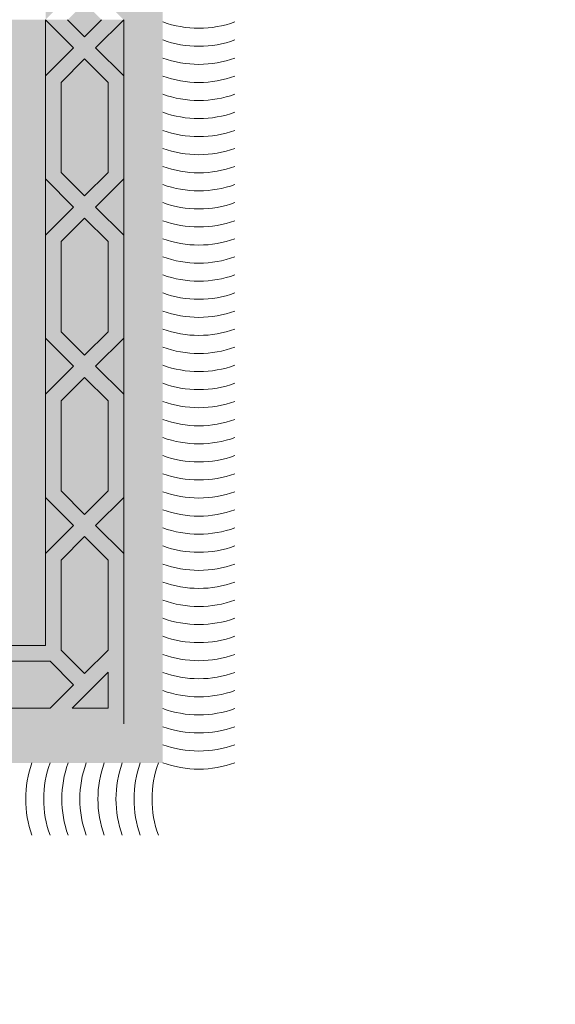
# Model space of a CAD drawing. Units: inches. Extents: x 844 to 2234, y 346 to 1084.
# Tile 12 of 93: x 1127.54 to 1136.28, y 680.17 to 696.22. Entities that reach past the tile are written whole.
import ezdxf

# ---------------------------------------------------------------- set-up
doc = ezdxf.new("R2010")
doc.units = ezdxf.units.IN
doc.header["$MEASUREMENT"] = 0
for name, color, linetype, lineweight in [('A-ANNO-DIMS', 2, 'Continuous', 18), ('furniture', 8, 'Continuous', 18), ('RA-AP-01$0$INT', 35, 'Continuous', 5)]:
    doc.layers.add(name, color=color, linetype=linetype, lineweight=lineweight)
doc.layers.add('RA-AP-01$0$FURN', color=3, linetype='Continuous')
doc.styles.get("Standard").update_dxf_attribs({"font": 'arial.ttf'})
doc.dimstyles.get("Standard").update_dxf_attribs({"dimtxt": 6, "dimasz": 3, "dimexe": 0.18, "dimexo": 0.0625, "dimgap": 0.09, "dimtad": 0, "dimtih": 1, "dimtoh": 1, "dimdec": 1, "dimzin": 0, "dimdsep": 46, "dimlunit": 3, "dimtxsty": 'Standard', "dimblk": 'ARCHTICK', "dimcen": 0.09, "dimadec": 0, "dimazin": 0, "dimtfac": 1, "dimtdec": 1, "dimtofl": 0, "dimtmove": 0, "dimatfit": 3, "dimfxl": 1, "dimtolj": 1, "dimtzin": 0, "dimarcsym": 0})

# ---------------------------------------------------------------- blocks, each defined once
blk = doc.blocks.new('A$C18D01794')
at = {"layer": 'RA-AP-01$0$INT'}
h = blk.add_hatch(color=256, dxfattribs=at)
h.paths.add_polyline_path([(4.3552, -6.1567), (4.3552, -8.0567), (5.4552, -8.0567), (5.4552, -6.1567)])
h.paths.add_polyline_path([(4.4052, -8.0067), (4.4052, -6.2067), (5.4052, -6.2067), (5.4052, -8.0067)], flags=16)
h = blk.add_hatch(color=256, dxfattribs=at)
h.paths.add_polyline_path([(4.4693, -7.0709), (4.5052, -7.035), (4.5052, -7.1067)])
h.paths.add_polyline_path([(4.4552, -7.085), (4.4769, -7.1067), (4.4335, -7.1067)])
h.paths.add_polyline_path([(4.4052, -7.035), (4.4411, -7.0709), (4.4052, -7.1067)])
h.paths.add_polyline_path([(4.4252, -6.9115), (4.4552, -6.8815), (4.4852, -6.9115), (4.4852, -7.0267), (4.4552, -7.0567), (4.4252, -7.0267)])
h.paths.add_polyline_path([(4.5052, -6.8315), (4.5052, -6.9032), (4.4693, -6.8673)])
h.paths.add_polyline_path([(4.4252, -6.7079), (4.4552, -6.6779), (4.4852, -6.7079), (4.4852, -6.8232), (4.4552, -6.8532), (4.4252, -6.8232)])
h.paths.add_polyline_path([(4.4252, -6.5044), (4.4552, -6.4744), (4.4852, -6.5044), (4.4852, -6.6196), (4.4552, -6.6496), (4.4252, -6.6196)])
h.paths.add_polyline_path([(4.4693, -6.6638), (4.5052, -6.6279), (4.5052, -6.6996)])
h.paths.add_polyline_path([(4.4052, -6.6279), (4.4411, -6.6638), (4.4052, -6.6996)])
h.paths.add_polyline_path([(4.4052, -6.4244), (4.4411, -6.4602), (4.4052, -6.4961)])
h.paths.add_polyline_path([(4.4693, -6.4602), (4.5052, -6.4244), (4.5052, -6.4961)])
h.paths.add_polyline_path([(4.4252, -6.3009), (4.4552, -6.2709), (4.4852, -6.3009), (4.4852, -6.4161), (4.4552, -6.4461), (4.4252, -6.4161)])
h.paths.add_polyline_path([(4.4252, -6.2267), (4.4711, -6.2267), (4.4252, -6.2726)])
h.paths.add_polyline_path([(4.4993, -6.2267), (4.6361, -6.2267), (4.6661, -6.2567), (4.6361, -6.2867), (4.4993, -6.2867), (4.4693, -6.2567)])
h.paths.add_polyline_path([(4.6802, -6.2709), (4.7161, -6.3067), (4.6443, -6.3067)])
h.paths.add_polyline_path([(4.6443, -6.2067), (4.7161, -6.2067), (4.6802, -6.2426)])
h.paths.add_polyline_path([(4.7243, -6.2267), (4.8611, -6.2267), (4.8911, -6.2567), (4.8611, -6.2867), (4.7243, -6.2867), (4.6943, -6.2567)])
h.paths.add_polyline_path([(4.9052, -6.2709), (4.9411, -6.3067), (4.8693, -6.3067)])
h.paths.add_polyline_path([(4.8693, -6.2067), (4.9411, -6.2067), (4.9052, -6.2426)])
h.paths.add_polyline_path([(4.9493, -6.2267), (5.0861, -6.2267), (5.1161, -6.2567), (5.0861, -6.2867), (4.9493, -6.2867), (4.9193, -6.2567)])
h.paths.add_polyline_path([(5.1302, -6.2709), (5.1661, -6.3067), (5.0943, -6.3067)])
h.paths.add_polyline_path([(5.0943, -6.2067), (5.1661, -6.2067), (5.1302, -6.2426)])
h.paths.add_polyline_path([(5.1743, -6.2267), (5.3111, -6.2267), (5.3411, -6.2567), (5.3111, -6.2867), (5.1743, -6.2867), (5.1443, -6.2567)])
h.paths.add_polyline_path([(5.3252, -6.3009), (5.3552, -6.2709), (5.3852, -6.3009), (5.3852, -6.4161), (5.3552, -6.4461), (5.3252, -6.4161)])
h.paths.add_polyline_path([(5.3393, -6.2267), (5.3852, -6.2267), (5.3852, -6.2726)])
h.paths.add_polyline_path([(5.3252, -6.5044), (5.3552, -6.4744), (5.3852, -6.5044), (5.3852, -6.6196), (5.3552, -6.6496), (5.3252, -6.6196)])
h.paths.add_polyline_path([(5.3052, -6.4244), (5.3411, -6.4602), (5.3052, -6.4961)])
h.paths.add_polyline_path([(5.3693, -6.4602), (5.4052, -6.4244), (5.4052, -6.4961)])
h.paths.add_polyline_path([(5.4052, -6.6279), (5.4052, -6.6996), (5.3693, -6.6638)])
h.paths.add_polyline_path([(5.3052, -6.6279), (5.3411, -6.6638), (5.3052, -6.6996)])
h.paths.add_polyline_path([(5.3252, -6.7079), (5.3552, -6.6779), (5.3852, -6.7079), (5.3852, -6.8232), (5.3552, -6.8532), (5.3252, -6.8232)])
h.paths.add_polyline_path([(5.3052, -6.8315), (5.3411, -6.8673), (5.3052, -6.9032)])
h.paths.add_polyline_path([(5.3252, -6.9115), (5.3552, -6.8815), (5.3852, -6.9115), (5.3852, -7.0267), (5.3552, -7.0567), (5.3252, -7.0267)])
h.paths.add_polyline_path([(5.4046, -6.8321, 0.001218), (5.4052, -6.8323), (5.4052, -6.9032), (5.3693, -6.8673)])
h.paths.add_polyline_path([(5.3693, -7.0709), (5.4052, -7.035), (5.4052, -7.1067)])
h.paths.add_polyline_path([(5.3552, -7.085), (5.3769, -7.1067), (5.3335, -7.1067)])
h.paths.add_polyline_path([(5.3052, -7.035), (5.3411, -7.0709), (5.3052, -7.1067)])
h = blk.add_hatch(color=256, dxfattribs=at)
h.paths.add_polyline_path([(4.5052, -6.6279), (4.4693, -6.6638), (4.5052, -6.6996), (4.5052, -6.8315), (4.4693, -6.8673), (4.5052, -6.9032), (4.5052, -7.035), (4.4693, -7.0709), (4.5052, -7.1067), (4.4769, -7.1067), (4.4552, -7.085), (4.4335, -7.1067), (4.4052, -7.1067), (4.4411, -7.0709), (4.4052, -7.035), (4.4052, -6.9032), (4.4411, -6.8673), (4.4052, -6.8315), (4.4052, -6.6996), (4.4411, -6.6638), (4.4052, -6.6279), (4.4052, -6.4961), (4.4411, -6.4602), (4.4052, -6.4244), (4.4052, -6.2067), (4.6443, -6.2067), (4.6802, -6.2426), (4.7161, -6.2067), (4.8693, -6.2067), (4.9052, -6.2426), (4.9411, -6.2067), (5.0943, -6.2067), (5.1302, -6.2426), (5.1661, -6.2067), (5.4052, -6.2067), (5.4052, -6.4244), (5.3693, -6.4602), (5.4052, -6.4961), (5.4052, -6.6279), (5.3693, -6.6638), (5.4052, -6.6996), (5.4052, -6.8315), (5.3693, -6.8673), (5.4052, -6.9032), (5.4052, -7.035), (5.3693, -7.0709), (5.4052, -7.1067), (5.3769, -7.1067), (5.3552, -7.085), (5.3335, -7.1067), (5.3052, -7.1067), (5.3411, -7.0709), (5.3052, -7.035), (5.3052, -6.9032), (5.3411, -6.8673), (5.3052, -6.8315), (5.3052, -6.6996), (5.3411, -6.6638), (5.3052, -6.6279), (5.3052, -6.4961), (5.3411, -6.4602), (5.3052, -6.4244), (5.3052, -6.3067), (5.1661, -6.3067), (5.1302, -6.2709), (5.0943, -6.3067), (4.9411, -6.3067), (4.9052, -6.2709), (4.8693, -6.3067), (4.7161, -6.3067), (4.6802, -6.2709), (4.6443, -6.3067), (4.5052, -6.3067), (4.5052, -6.4244), (4.4693, -6.4602), (4.5052, -6.4961)])
h.paths.add_polyline_path([(4.4852, -6.5044), (4.4552, -6.4744), (4.4252, -6.5044), (4.4252, -6.6196), (4.4552, -6.6496), (4.4852, -6.6196)], flags=16)
h.paths.add_polyline_path([(4.4552, -6.4461), (4.4852, -6.4161), (4.4852, -6.3009), (4.4552, -6.2709), (4.4252, -6.3009), (4.4252, -6.4161)], flags=16)
h.paths.add_polyline_path([(4.4552, -6.6779), (4.4252, -6.7079), (4.4252, -6.8232), (4.4552, -6.8532), (4.4852, -6.8232), (4.4852, -6.7079)], flags=16)
h.paths.add_polyline_path([(4.4993, -6.2867), (4.6361, -6.2867), (4.6661, -6.2567), (4.6361, -6.2267), (4.4993, -6.2267), (4.4693, -6.2567)], flags=16)
h.paths.add_polyline_path([(4.4252, -6.2726), (4.4711, -6.2267), (4.4252, -6.2267)], flags=16)
h.paths.add_polyline_path([(4.4552, -6.8815), (4.4252, -6.9115), (4.4252, -7.0267), (4.4552, -7.0567), (4.4852, -7.0267), (4.4852, -6.9115)], flags=16)
h.paths.add_polyline_path([(4.7243, -6.2867), (4.8611, -6.2867), (4.8911, -6.2567), (4.8611, -6.2267), (4.7243, -6.2267), (4.6943, -6.2567)], flags=16)
h.paths.add_polyline_path([(4.9193, -6.2567), (4.9493, -6.2867), (5.0861, -6.2867), (5.1161, -6.2567), (5.0861, -6.2267), (4.9493, -6.2267)], flags=16)
h.paths.add_polyline_path([(5.1443, -6.2567), (5.1743, -6.2867), (5.3111, -6.2867), (5.3411, -6.2567), (5.3111, -6.2267), (5.1743, -6.2267)], flags=16)
h.paths.add_polyline_path([(5.3252, -6.6196), (5.3552, -6.6496), (5.3852, -6.6196), (5.3852, -6.5044), (5.3552, -6.4744), (5.3252, -6.5044)], flags=16)
h.paths.add_polyline_path([(5.3252, -6.4161), (5.3552, -6.4461), (5.3852, -6.4161), (5.3852, -6.3009), (5.3552, -6.2709), (5.3252, -6.3009)], flags=16)
h.paths.add_polyline_path([(5.3252, -6.7079), (5.3252, -6.8232), (5.3552, -6.8532), (5.3852, -6.8232), (5.3852, -6.7079), (5.3552, -6.6779)], flags=16)
h.paths.add_polyline_path([(5.3252, -6.9115), (5.3252, -7.0267), (5.3552, -7.0567), (5.3852, -7.0267), (5.3852, -6.9115), (5.3552, -6.8815)], flags=16)
h.paths.add_polyline_path([(5.3393, -6.2267), (5.3852, -6.2726), (5.3852, -6.2267)], flags=16)
blk.add_hatch(color=256, dxfattribs=at).paths.add_polyline_path([(4.5052, -6.3067), (5.3052, -6.3067), (5.3052, -7.1067), (5.2552, -7.1067), (5.2552, -6.3567), (4.5552, -6.3567), (4.5552, -7.1067), (4.5052, -7.1067)])
h = blk.add_hatch(color=256, dxfattribs=at)
h.paths.add_polyline_path([(4.4693, -7.1426), (4.5052, -7.1784), (4.5052, -7.1067)])
h.paths.add_polyline_path([(4.4552, -7.1284), (4.4769, -7.1067), (4.4335, -7.1067)])
h.paths.add_polyline_path([(4.4052, -7.1784), (4.4411, -7.1426), (4.4052, -7.1067)])
h.paths.add_polyline_path([(4.4252, -7.302), (4.4552, -7.332), (4.4852, -7.302), (4.4852, -7.1867), (4.4552, -7.1567), (4.4252, -7.1867)])
h.paths.add_polyline_path([(4.5052, -7.382), (4.5052, -7.3102), (4.4693, -7.3461)])
h.paths.add_polyline_path([(4.4252, -7.5055), (4.4552, -7.5355), (4.4852, -7.5055), (4.4852, -7.3902), (4.4552, -7.3602), (4.4252, -7.3902)])
h.paths.add_polyline_path([(4.4252, -7.709), (4.4552, -7.739), (4.4852, -7.709), (4.4852, -7.5938), (4.4552, -7.5638), (4.4252, -7.5938)])
h.paths.add_polyline_path([(4.4693, -7.5496), (4.5052, -7.5855), (4.5052, -7.5138)])
h.paths.add_polyline_path([(4.4052, -7.5855), (4.4411, -7.5496), (4.4052, -7.5138)])
h.paths.add_polyline_path([(4.4052, -7.789), (4.4411, -7.7532), (4.4052, -7.7173)])
h.paths.add_polyline_path([(4.4693, -7.7532), (4.5052, -7.789), (4.5052, -7.7173)])
h.paths.add_polyline_path([(4.4252, -7.9126), (4.4552, -7.9426), (4.4852, -7.9126), (4.4852, -7.7973), (4.4552, -7.7673), (4.4252, -7.7973)])
h.paths.add_polyline_path([(4.4252, -7.9867), (4.4711, -7.9867), (4.4252, -7.9409)])
h.paths.add_polyline_path([(4.4993, -7.9867), (4.6361, -7.9867), (4.6661, -7.9567), (4.6361, -7.9267), (4.4993, -7.9267), (4.4693, -7.9567)])
h.paths.add_polyline_path([(4.6802, -7.9426), (4.7161, -7.9067), (4.6443, -7.9067)])
h.paths.add_polyline_path([(4.6443, -8.0067), (4.7161, -8.0067), (4.6802, -7.9709)])
h.paths.add_polyline_path([(4.7243, -7.9867), (4.8611, -7.9867), (4.8911, -7.9567), (4.8611, -7.9267), (4.7243, -7.9267), (4.6943, -7.9567)])
h.paths.add_polyline_path([(4.9052, -7.9426), (4.9411, -7.9067), (4.8693, -7.9067)])
h.paths.add_polyline_path([(4.8693, -8.0067), (4.9411, -8.0067), (4.9052, -7.9709)])
h.paths.add_polyline_path([(4.9493, -7.9867), (5.0861, -7.9867), (5.1161, -7.9567), (5.0861, -7.9267), (4.9493, -7.9267), (4.9193, -7.9567)])
h.paths.add_polyline_path([(5.1302, -7.9426), (5.1661, -7.9067), (5.0943, -7.9067)])
h.paths.add_polyline_path([(5.0943, -8.0067), (5.1661, -8.0067), (5.1302, -7.9709)])
h.paths.add_polyline_path([(5.1743, -7.9867), (5.3111, -7.9867), (5.3411, -7.9567), (5.3111, -7.9267), (5.1743, -7.9267), (5.1443, -7.9567)])
h.paths.add_polyline_path([(5.3252, -7.9126), (5.3552, -7.9426), (5.3852, -7.9126), (5.3852, -7.7973), (5.3552, -7.7673), (5.3252, -7.7973)])
h.paths.add_polyline_path([(5.3393, -7.9867), (5.3852, -7.9867), (5.3852, -7.9409)])
h.paths.add_polyline_path([(5.3252, -7.709), (5.3552, -7.739), (5.3852, -7.709), (5.3852, -7.5938), (5.3552, -7.5638), (5.3252, -7.5938)])
h.paths.add_polyline_path([(5.3052, -7.789), (5.3411, -7.7532), (5.3052, -7.7173)])
h.paths.add_polyline_path([(5.3693, -7.7532), (5.4052, -7.789), (5.4052, -7.7173)])
h.paths.add_polyline_path([(5.4052, -7.5855), (5.4052, -7.5138), (5.3693, -7.5496)])
h.paths.add_polyline_path([(5.3052, -7.5855), (5.3411, -7.5496), (5.3052, -7.5138)])
h.paths.add_polyline_path([(5.3252, -7.5055), (5.3552, -7.5355), (5.3852, -7.5055), (5.3852, -7.3902), (5.3552, -7.3602), (5.3252, -7.3902)])
h.paths.add_polyline_path([(5.3052, -7.382), (5.3411, -7.3461), (5.3052, -7.3102)])
h.paths.add_polyline_path([(5.3252, -7.302), (5.3552, -7.332), (5.3852, -7.302), (5.3852, -7.1867), (5.3552, -7.1567), (5.3252, -7.1867)])
h.paths.add_polyline_path([(5.4046, -7.3813, -0.001218), (5.4052, -7.3811), (5.4052, -7.3102), (5.3693, -7.3461)])
h.paths.add_polyline_path([(5.3693, -7.1426), (5.4052, -7.1784), (5.4052, -7.1067)])
h.paths.add_polyline_path([(5.3552, -7.1284), (5.3769, -7.1067), (5.3335, -7.1067)])
h.paths.add_polyline_path([(5.3052, -7.1784), (5.3411, -7.1426), (5.3052, -7.1067)])
for p, q in [((5.1743, -6.2267), (5.3111, -6.2267)), ((5.3111, -6.2267), (5.3411, -6.2567)), ((5.3393, -6.2267), (5.3852, -6.2726)), ((5.3393, -6.2267), (5.3852, -6.2267)), ((5.3852, -6.2726), (5.3852, -6.2267)), ((5.3111, -6.2867), (5.3411, -6.2567)), ((5.3252, -6.3009), (5.3552, -6.2709)), ((5.3852, -6.3009), (5.3552, -6.2709)), ((5.1743, -6.2867), (5.3111, -6.2867)), ((5.3252, -6.3009), (5.3252, -6.4161)), ((5.3852, -6.4161), (5.3852, -6.3009)), ((5.3552, -6.4461), (5.3252, -6.4161)), ((5.3552, -6.4461), (5.3852, -6.4161)), ((5.3411, -6.4602), (5.3052, -6.4244)), ((5.3693, -6.4602), (5.4052, -6.4244)), ((5.3052, -6.4961), (5.3411, -6.4602)), ((5.4052, -6.4961), (5.3693, -6.4602)), ((5.3252, -6.5044), (5.3552, -6.4744)), ((5.3852, -6.5044), (5.3552, -6.4744)), ((5.3252, -6.6196), (5.3252, -6.5044)), ((5.3852, -6.6196), (5.3852, -6.5044)), ((5.3252, -6.6196), (5.3552, -6.6496)), ((5.3852, -6.6196), (5.3552, -6.6496)), ((5.3052, -6.6279), (5.3411, -6.6638)), ((5.4052, -6.6279), (5.3693, -6.6638)), ((5.3052, -6.6996), (5.3411, -6.6638)), ((5.4052, -6.6996), (5.3693, -6.6638)), ((5.3252, -6.7079), (5.3552, -6.6779)), ((5.3852, -6.7079), (5.3552, -6.6779)), ((5.3252, -6.8232), (5.3252, -6.7079)), ((5.3852, -6.8232), (5.3852, -6.7079)), ((5.3052, -6.8315), (5.3411, -6.8673)), ((5.3252, -6.8232), (5.3552, -6.8532)), ((5.3852, -6.8232), (5.3552, -6.8532)), ((5.4052, -6.8315), (5.3693, -6.8673)), ((5.3052, -6.9032), (5.3411, -6.8673)), ((5.4052, -6.9032), (5.3693, -6.8673)), ((5.3252, -6.9115), (5.3552, -6.8815)), ((5.3852, -6.9115), (5.3552, -6.8815)), ((5.3252, -6.9115), (5.3252, -7.0267)), ((5.3852, -6.9115), (5.3852, -7.0267)), ((5.3052, -7.035), (5.3411, -7.0709)), ((5.3252, -7.0267), (5.3552, -7.0567)), ((5.3852, -7.0267), (5.3552, -7.0567)), ((5.4052, -7.035), (5.3693, -7.0709)), ((5.3411, -7.0709), (5.3052, -7.1067)), ((5.3693, -7.0709), (5.4052, -7.1067)), ((5.3552, -7.085), (5.3335, -7.1067)), ((5.3552, -7.085), (5.3769, -7.1067))]:
    blk.add_line(p, q, dxfattribs=at)
for points in [[(5.4052, -7.1067), (5.4052, -6.2067)], [(5.3052, -7.1067), (5.3052, -6.3067), (4.5052, -6.3067), (4.5052, -7.1067)]]:
    blk.add_lwpolyline(points, dxfattribs=at)
for centre, start, end in [((5.4162, -6.1105), 160.2038, 199.7962), ((5.4393, -6.1105), 160.2038, 199.7962), ((5.4624, -6.1105), 160.2038, 199.7962), ((5.4855, -6.1105), 160.2038, 199.7962), ((5.5086, -6.1105), 160.2038, 199.7962), ((5.5317, -6.1105), 160.2038, 199.7962), ((5.5548, -6.1105), 160.2038, 199.7962), ((5.5779, -6.1105), 160.2038, 199.7962), ((5.5014, -6.2852), 70.2038, 109.7962), ((5.5014, -6.3083), 70.2038, 109.7962), ((5.5014, -6.3314), 70.2038, 109.7962), ((5.5014, -6.3545), 70.2038, 109.7962), ((5.5014, -6.3776), 70.2038, 109.7962), ((5.5014, -6.4007), 70.2038, 109.7962), ((5.5014, -6.4238), 70.2038, 109.7962), ((5.5014, -6.4469), 70.2038, 109.7962), ((5.5014, -6.47), 70.2038, 109.7962), ((5.5014, -6.4931), 70.2038, 109.7962), ((5.5014, -6.5162), 70.2038, 109.7962), ((5.5014, -6.5393), 70.2038, 109.7962), ((5.5014, -6.5624), 70.2038, 109.7962), ((5.5014, -6.5855), 70.2038, 109.7962), ((5.5014, -6.6086), 70.2038, 109.7962), ((5.5014, -6.6317), 70.2038, 109.7962), ((5.5014, -6.6548), 70.2038, 109.7962), ((5.5014, -6.6779), 70.2038, 109.7962), ((5.5014, -6.701), 70.2038, 109.7962), ((5.5014, -6.7241), 70.2038, 109.7962), ((5.5014, -6.7472), 70.2038, 109.7962), ((5.5014, -6.7703), 70.2038, 109.7962), ((5.5014, -6.7934), 70.2038, 109.7962), ((5.5014, -6.7934), 70.2038, 109.7962), ((5.5014, -6.8165), 70.2038, 109.7962), ((5.5014, -6.8396), 70.2038, 109.7962), ((5.5014, -6.8627), 70.2038, 109.7962), ((5.5014, -6.8858), 70.2038, 109.7962), ((5.5014, -6.9089), 70.2038, 109.7962), ((5.5014, -6.932), 70.2038, 109.7962), ((5.5014, -6.9551), 70.2038, 109.7962), ((5.5014, -6.9782), 70.2038, 109.7962), ((5.5014, -7.0013), 70.2038, 109.7962), ((5.5014, -7.0244), 70.2038, 109.7962), ((5.5014, -7.0475), 70.2038, 109.7962), ((5.5014, -7.0706), 70.2038, 109.7962), ((5.5014, -7.0937), 70.2038, 109.7962), ((5.5014, -7.1168), 70.2038, 109.7962), ((5.5014, -7.1399), 70.2038, 109.7962), ((5.5014, -7.163), 70.2038, 109.7962), ((5.5014, -7.1861), 70.2038, 109.7962), ((5.5014, -7.2092), 70.2038, 109.7962), ((5.5014, -7.2323), 70.2038, 109.7962)]:
    blk.add_arc(centre, 0.1364, start, end, dxfattribs=at)
blk = doc.blocks.new('A$C5D2F253E')
at = {"layer": 'RA-AP-01$0$FURN', "xscale": -0.7999999999883585, "yscale": 0.7999999999883585, "zscale": 0.8, "rotation": 90}
blk.add_blockref('A$C18D01794', (-5.6878, 4.7579), dxfattribs=at)
blk = doc.blocks.new('_ArchTick')
at = {"color": 0, "linetype": 'ByBlock', "const_width": 0.15}
blk.add_lwpolyline([(-0.5, -0.5), (0.5, 0.5)], dxfattribs=at)
blk = doc.blocks.new('*D144')
at = {"layer": 'A-ANNO-DIMS', "color": 0, "lineweight": -2, "transparency": 16777216}
for p, q in [((1096.616, 439.373), (1096.616, 1074.743)), ((1143.116, 492.373), (1143.116, 1074.743)), ((1096.616, 1074.563), (1102.482, 1074.563)), ((1143.116, 1074.563), (1137.25, 1074.563))]:
    blk.add_line(p, q, dxfattribs=at)
at = {"layer": 'Defpoints', "color": 0, "transparency": 16777216}
for p in [(1143.116, 1074.563), (1143.116, 492.311), (1096.616, 439.311)]:
    blk.add_point(p, dxfattribs=at)
at = {"layer": 'A-ANNO-DIMS', "color": 0, "lineweight": -2, "transparency": 16777216, "xscale": 3, "yscale": 3, "zscale": 3, "rotation": 180}
blk.add_blockref('_ArchTick', (1096.616, 1074.563), dxfattribs=at)
at = {"layer": 'A-ANNO-DIMS', "color": 0, "lineweight": -2, "transparency": 16777216, "xscale": 3, "yscale": 3, "zscale": 3}
blk.add_blockref('_ArchTick', (1143.116, 1074.563), dxfattribs=at)
at = {"layer": 'A-ANNO-DIMS', "color": 0, "transparency": 16777216, "insert": (1119.866, 1074.563), "char_height": 6, "attachment_point": 5}
blk.add_mtext('\\A1;3\'-10 1/2"', dxfattribs=at)

msp = doc.modelspace()

# ---------------------------------------------------------------- block references
at = {"layer": 'furniture', "xscale": 15.94108302203742, "yscale": 15.94108302203742, "zscale": 15.94108302203742, "rotation": 90}
msp.add_blockref('A$C5D2F253E', (1136.148, 696.258), dxfattribs=at)

# ---------------------------------------------------------------- dimensions: what is measured, and where the dimension line sits
at = {"layer": 'A-ANNO-DIMS'}
dim = msp.add_linear_dim(base=(1143.116, 1074.563), p1=(1096.616, 439.311), p2=(1143.116, 492.311), dimstyle='Standard', override={"dimdec": 1, "dimlfac": 1, "dimrnd": 0, "dimzin": 1, "dimdsep": 46, "dimlunit": 4, "dimfrac": 2}, dxfattribs=at)
dim.commit()
dim.dimension.update_dxf_attribs({"geometry": '*D144', "text_midpoint": (1119.866, 1074.563)})

doc.saveas('drawing.dxf')
